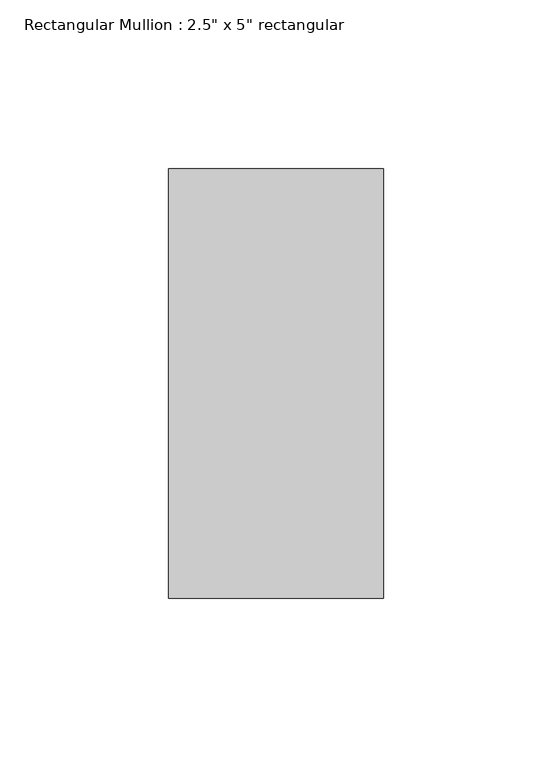
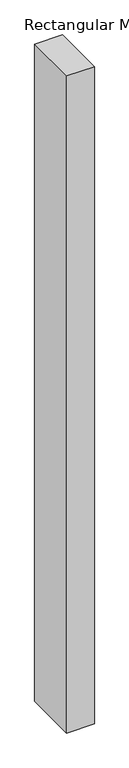
"""IFC4 building model written with IfcOpenShell, lengths in millimetres: member geometry."""

from ifc_helpers import new_model, si_unit, frame, origin, place, context, project, spatial, polyline, outline, extrude, source, transform, mapped, element, save


def member_b315899a(model_context):
    return source(origin(), model_context, "Body", "SweptSolid", [
        extrude(outline(polyline([(0.0, 63.5), (0.0, -63.5), (-63.5, -63.5), (-63.5, 63.5), (0.0, 63.5)])), frame((0.0, 0.0, -1594.6445261), z_axis=(0.0, 0.0, 1.0), x_axis=(1.0, 0.0, 0.0)), (0.0, 0.0, 1.0), 1594.6445261),
    ])


if __name__ == "__main__":
    model = new_model("IFC4")
    model_context = context("Model", 3, world=origin())
    ifc_project = project(units=[si_unit("LENGTHUNIT", "METRE", prefix="MILLI")], contexts=[model_context])
    site = spatial("IfcSite", under=ifc_project)
    building = spatial("IfcBuilding", under=site)
    placement = place(None, origin())
    member_shape = member_b315899a(model_context)
    element("IfcMember", 1, ObjectType="Rectangular Mullion : 2.5\" x 5\" rectangular", at=placement, inside=building, context=model_context, shape_type="MappedRepresentation", body=[
        mapped(member_shape, transform((0.0, 0.0, 0.0), x_axis=(1.0, 0.0, 0.0), y_axis=(0.0, 1.0, 0.0), z_axis=(0.0, 0.0, 1.0))),
    ])
    save(model, "model.ifc")

# Revit data of these elements
# Type "Rectangular Mullion : 2.5\" x 5\" rectangular"
#   built-in parameter 1007304 = 0.416667 (stored number, unit not read)
#   built-in parameter 1007301 = 0.104167 (stored number, unit not read)
#   built-in parameter 1007300 = 0.104167 (stored number, unit not read)
# Element 1 (IfcMember, "Rectangular Mullion : 2.5\" x 5\" rectangular")
#   Materials on its faces: "Aluminum"
# Materials
#   "Aluminum": class "Metal", colour RGB 247 247 247, transparency 0, Description = "Aluminum 6061", Cost = 0
